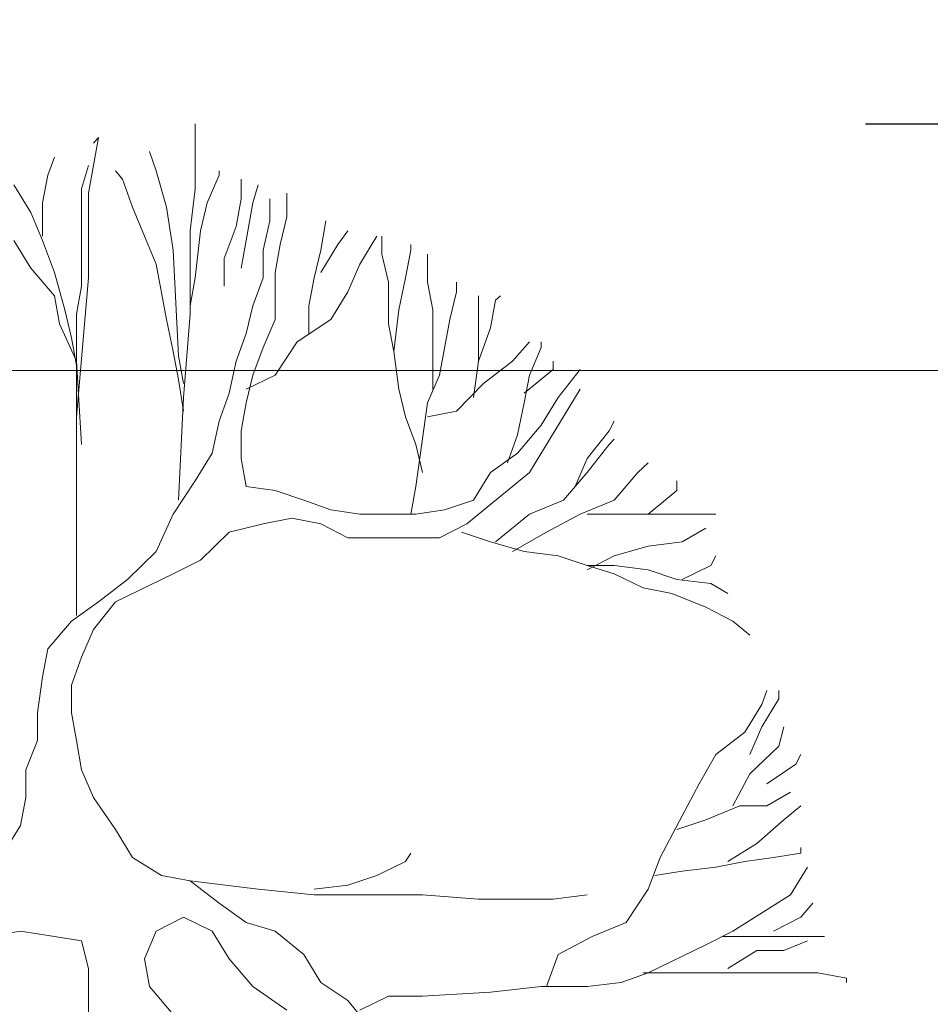
# Model space of a CAD drawing. Units: millimetres. Extents: x 595116 to 630915, y 909473 to 920225.
# Tile 53 of 134: x 629559 to 629589, y 919281 to 919314. Entities that reach past the tile are written whole.
import ezdxf

# ---------------------------------------------------------------- set-up
doc = ezdxf.new("R2010")
doc.units = ezdxf.units.MM
doc.layers.add('Dimension', color=3, linetype='Continuous', lineweight=18)
doc.layers.add('L-PLNT', color=85, linetype='Continuous', lineweight=13)
doc.styles.get("Standard").update_dxf_attribs({"font": 'arial.ttf'})
doc.dimstyles.new('ISO-25', dxfattribs={"dimtxt": 9, "dimasz": 6, "dimexe": 1.25, "dimexo": 0.625, "dimtad": 1, "dimlunit": 4, "dimtxsty": 'Standard', "dimcen": 2.5, "dimadec": 0, "dimazin": 0, "dimtfac": 1, "dimtmove": 0, "dimatfit": 3, "dimfxl": 1, "dimarcsym": 0})

# ---------------------------------------------------------------- blocks, each defined once
blk = doc.blocks.new('A$C143125F4')
for p, q in [((2.883, 4.8338), (2.883, 5.0443)), ((2.5383, 4.8203), (2.5711, 4.9995)), ((2.5711, 4.9995), (2.5547, 4.9816)), ((2.7571, 4.892), (2.7353, 4.9547)), ((2.407, 4.8786), (2.4289, 4.9368)), ((2.5164, 4.8338), (2.5383, 4.9099)), ((2.6477, 4.8651), (2.6259, 4.892)), ((2.79, 4.7755), (2.7571, 4.892)), ((2.9596, 4.8786), (2.9596, 4.892)), ((2.3906, 4.789), (2.407, 4.8786)), ((2.6806, 4.7755), (2.6477, 4.8651)), ((2.9213, 4.789), (2.9596, 4.8786)), ((3.0307, 4.8024), (3.0307, 4.8651)), ((2.3523, 4.7576), (2.2976, 4.8472)), ((2.5164, 4.5202), (2.5164, 4.8338)), ((2.8666, 4.6994), (2.883, 4.8338)), ((3.069, 4.789), (3.0854, 4.8472)), ((2.5383, 4.5471), (2.5383, 4.8203)), ((3.0143, 4.7128), (3.0307, 4.8024)), ((3.1237, 4.7307), (3.1237, 4.8024)), ((3.1784, 4.7442), (3.1784, 4.8203)), ((2.3906, 4.6814), (2.3906, 4.789)), ((2.7189, 4.6814), (2.6806, 4.7755)), ((2.8119, 4.6367), (2.79, 4.7755)), ((2.8994, 4.6994), (2.9213, 4.789)), ((3.0471, 4.668), (3.069, 4.789)), ((2.3906, 4.668), (2.3523, 4.7576)), ((3.1018, 4.6367), (3.1237, 4.7307)), ((3.1565, 4.6546), (3.1784, 4.7442)), ((3.2878, 4.6367), (3.3042, 4.7307)), ((2.8666, 4.4306), (2.8666, 4.6994)), ((2.883, 4.5471), (2.8994, 4.6994)), ((2.976, 4.6098), (3.0143, 4.7128)), ((3.3425, 4.6546), (3.3753, 4.6994)), ((2.3523, 4.5784), (2.2976, 4.668)), ((2.4289, 4.565), (2.3906, 4.668)), ((2.7571, 4.5919), (2.7189, 4.6814)), ((3.0307, 4.5784), (3.0471, 4.668)), ((3.4136, 4.5919), (3.4683, 4.6814)), ((3.4847, 4.6232), (3.4847, 4.6814)), ((2.8283, 4.2962), (2.8119, 4.6367)), ((3.1018, 4.5471), (3.1018, 4.6367)), ((3.1401, 4.565), (3.1565, 4.6546)), ((3.2659, 4.5471), (3.2878, 4.6367)), ((3.2878, 4.565), (3.3425, 4.6546)), ((3.5613, 4.5471), (3.5777, 4.6367)), ((3.5777, 4.6367), (3.5777, 4.6546)), ((2.976, 4.5202), (2.976, 4.6098)), ((3.5066, 4.5336), (3.4847, 4.6232)), ((3.6324, 4.5336), (3.6324, 4.6232)), ((2.4289, 4.4888), (2.3523, 4.5784)), ((2.79, 4.4127), (2.7571, 4.5919)), ((3.3753, 4.5023), (3.4136, 4.5919)), ((2.4617, 4.444), (2.4289, 4.565)), ((2.5, 4.0991), (2.5383, 4.5471)), ((2.8666, 4.4575), (2.883, 4.5471)), ((3.069, 4.4575), (3.1018, 4.5471)), ((3.1401, 4.4127), (3.1401, 4.565)), ((3.2495, 4.4575), (3.2659, 4.5471)), ((3.5394, 4.444), (3.5613, 4.5471)), ((2.5, 4.4306), (2.5164, 4.5202)), ((3.5066, 4.3992), (3.5066, 4.5336)), ((3.6488, 4.444), (3.6324, 4.5336)), ((3.7254, 4.5023), (3.7254, 4.5336)), ((2.4453, 4.3992), (2.4289, 4.4888)), ((3.3206, 4.4127), (3.3753, 4.5023)), ((3.7035, 4.4127), (3.7254, 4.5023)), ((3.7965, 4.2783), (3.7965, 4.4888)), ((3.8512, 4.4754), (3.8677, 4.4888)), ((3.0471, 4.3679), (3.069, 4.4575)), ((3.2495, 4.3679), (3.2495, 4.4575)), ((3.8348, 4.3858), (3.8512, 4.4754)), ((2.4836, 4.3544), (2.4617, 4.444)), ((2.5, 3.4584), (2.5, 4.4306)), ((2.8119, 4.3096), (2.79, 4.4127)), ((2.8447, 4.1618), (2.8666, 4.4306)), ((3.1018, 4.3231), (3.1401, 4.4127)), ((3.2112, 4.341), (3.3206, 4.4127)), ((3.523, 4.3096), (3.5394, 4.444)), ((3.6488, 4.1887), (3.6488, 4.444)), ((3.6707, 4.2335), (3.7035, 4.4127)), ((2.5, 4.2783), (2.4453, 4.3992)), ((3.523, 4.3096), (3.5066, 4.3992)), ((3.7965, 4.2783), (3.8348, 4.3858)), ((2.5, 4.2648), (2.4836, 4.3544)), ((3.0143, 4.2783), (3.0471, 4.3679)), ((3.069, 4.2335), (3.1018, 4.3231)), ((3.1401, 4.2335), (3.2112, 4.341)), ((3.906, 4.2783), (3.9607, 4.341)), ((3.9607, 4.2335), (3.999, 4.3231)), ((3.999, 4.3231), (3.999, 4.341)), ((2.8283, 4.22), (2.8119, 4.3096)), ((2.8447, 4.2066), (2.8283, 4.2962)), ((3.5394, 4.1887), (3.523, 4.3096)), ((2.5164, 4.0095), (2.5, 4.2783)), ((2.9924, 4.1752), (3.0143, 4.2783)), ((3.7801, 4.1618), (3.7965, 4.2783)), ((3.813, 4.2066), (3.906, 4.2783)), ((4.0372, 4.2514), (4.0372, 4.2783)), ((3.0471, 4.1887), (3.1401, 4.2335)), ((3.0471, 4.1439), (3.069, 4.2335)), ((3.6324, 4.1439), (3.6707, 4.2335)), ((3.9442, 4.1752), (4.0372, 4.2514)), ((3.9442, 4.1439), (3.9607, 4.2335)), ((4.1248, 4.2514), (4.0537, 4.1618)), ((2.8447, 4.117), (2.8283, 4.22)), ((3.7254, 4.117), (3.813, 4.2066)), ((2.8283, 3.8303), (2.8447, 4.1618)), ((2.9596, 4.0856), (2.9924, 4.1752)), ((3.5613, 4.0991), (3.5394, 4.1887)), ((3.9607, 3.9199), (4.1248, 4.1887)), ((4.0537, 4.1618), (3.999, 4.0722)), ((3.0307, 4.0543), (3.0471, 4.1439)), ((3.5941, 3.8751), (3.6324, 4.1439)), ((3.9224, 4.0408), (3.9442, 4.1439)), ((2.5, 3.996), (2.5, 4.0991)), ((3.5941, 4.0095), (3.5613, 4.0991)), ((3.6324, 4.0991), (3.7254, 4.117)), ((2.9377, 3.9826), (2.9596, 4.0856)), ((3.999, 4.0722), (3.9224, 3.9826)), ((4.2178, 4.0543), (4.2342, 4.0856)), ((3.0307, 3.9647), (3.0307, 4.0543)), ((3.8895, 3.9512), (3.9224, 4.0408)), ((4.1467, 3.9647), (4.2178, 4.0543)), ((3.616, 3.9199), (3.5941, 4.0095)), ((4.1467, 3.9199), (4.2178, 4.0095)), ((4.2178, 4.0095), (4.2342, 4.0274)), ((2.883, 3.893), (2.9377, 3.9826)), ((3.9224, 3.9826), (3.8348, 3.9199)), ((3.0471, 3.8751), (3.0307, 3.9647)), ((4.1084, 3.8751), (4.1467, 3.9647)), ((4.3108, 3.9199), (4.3436, 3.9512)), ((3.7583, 3.7541), (3.9607, 3.9199)), ((3.8348, 3.9199), (3.7801, 3.8303)), ((4.0701, 3.8303), (4.1467, 3.9199)), ((4.2342, 3.8303), (4.3108, 3.9199)), ((2.8119, 3.7855), (2.883, 3.893)), ((3.1401, 3.8616), (3.0471, 3.8751)), ((3.5777, 3.7855), (3.5941, 3.8751)), ((4.4366, 3.8616), (4.4366, 3.893)), ((3.2331, 3.8303), (3.1401, 3.8616)), ((4.3436, 3.7855), (4.4366, 3.8616)), ((3.3206, 3.7989), (3.2331, 3.8303)), ((3.7801, 3.8303), (3.6871, 3.7989)), ((3.9607, 3.7855), (4.0701, 3.8303)), ((4.1248, 3.7855), (4.2342, 3.8303)), ((2.7571, 3.6645), (2.8119, 3.7855)), ((3.4136, 3.7855), (3.3206, 3.7989)), ((3.5941, 3.7855), (3.4136, 3.7855)), ((3.6871, 3.7989), (3.5941, 3.7855)), ((3.8512, 3.6959), (3.9607, 3.7855)), ((4.0154, 3.7272), (4.1248, 3.7855)), ((4.1467, 3.7855), (4.5624, 3.7855)), ((2.9924, 3.7272), (3.1018, 3.7541)), ((3.1018, 3.7541), (3.1948, 3.772)), ((3.1948, 3.772), (3.2878, 3.7541)), ((3.2878, 3.7541), (3.3753, 3.7093)), ((3.6707, 3.7093), (3.7583, 3.7541)), ((2.8994, 3.6376), (2.9924, 3.7272)), ((3.7418, 3.7272), (3.8348, 3.6959)), ((3.906, 3.6645), (4.0154, 3.7272)), ((4.453, 3.6959), (4.5296, 3.7407)), ((3.3753, 3.7093), (3.6707, 3.7093)), ((3.8348, 3.6959), (3.9442, 3.6645)), ((4.2342, 3.6511), (4.3436, 3.6824)), ((4.3436, 3.6824), (4.453, 3.6959)), ((2.6641, 3.5749), (2.7571, 3.6645)), ((3.9442, 3.6645), (4.0537, 3.6511)), ((4.0537, 3.6511), (4.1467, 3.6197)), ((4.1467, 3.6063), (4.2342, 3.6511)), ((4.546, 3.6197), (4.5624, 3.6511)), ((2.8119, 3.5928), (2.8994, 3.6376)), ((4.1467, 3.6197), (4.2342, 3.5928)), ((4.1467, 3.6197), (4.2342, 3.6197)), ((4.2342, 3.6197), (4.3436, 3.6063)), ((4.453, 3.5749), (4.546, 3.6197)), ((2.6259, 3.5032), (2.8119, 3.5928)), ((4.2342, 3.5928), (4.3272, 3.548)), ((4.3436, 3.6063), (4.4366, 3.5749)), ((2.5711, 3.5032), (2.6641, 3.5749)), ((4.4366, 3.5749), (4.546, 3.5615)), ((4.546, 3.5615), (4.6007, 3.5301)), ((4.3272, 3.548), (4.4202, 3.5301)), ((4.4202, 3.5301), (4.5296, 3.4853)), ((2.4836, 3.4405), (2.5711, 3.5032)), ((2.5547, 3.4136), (2.6259, 3.5032)), ((4.5296, 3.4853), (4.6171, 3.4405)), ((2.407, 3.3509), (2.4836, 3.4405)), ((4.6171, 3.4405), (4.6718, 3.3957)), ((2.5164, 3.3241), (2.5547, 3.4136)), ((2.3906, 3.2613), (2.407, 3.3509)), ((2.4836, 3.2345), (2.5164, 3.3241)), ((2.3742, 3.1449), (2.3906, 3.2613)), ((2.4836, 3.1449), (2.4836, 3.2345)), ((4.7101, 3.1717), (4.7265, 3.2165)), ((4.7648, 3.1897), (4.7648, 3.2165)), ((4.7101, 3.1001), (4.7648, 3.1897)), ((2.3742, 3.0553), (2.3742, 3.1449)), ((2.5, 3.0553), (2.4836, 3.1449)), ((4.6554, 3.0821), (4.7101, 3.1717)), ((4.5624, 3.0105), (4.6554, 3.0821)), ((4.6718, 3.0105), (4.7101, 3.1001)), ((4.7648, 3.0373), (4.7812, 3.1001)), ((2.3359, 2.9612), (2.3742, 3.0553)), ((2.5164, 2.9612), (2.5, 3.0553)), ((4.6718, 2.9477), (4.7648, 3.0373)), ((4.5077, 2.9164), (4.5624, 3.0105)), ((4.8195, 2.9791), (4.8359, 3.0105)), ((2.3359, 2.8716), (2.3359, 2.9612)), ((2.5547, 2.8716), (2.5164, 2.9612)), ((4.7265, 2.9164), (4.8195, 2.9791)), ((4.6171, 2.8447), (4.6718, 2.9477)), ((4.453, 2.8133), (4.5077, 2.9164)), ((4.7265, 2.8447), (4.8031, 2.8895)), ((2.3195, 2.782), (2.3359, 2.8716)), ((2.6259, 2.7686), (2.5547, 2.8716)), ((4.5296, 2.7999), (4.639, 2.8447)), ((4.639, 2.8447), (4.7265, 2.8447)), ((4.7812, 2.7999), (4.8359, 2.8447)), ((4.3819, 2.679), (4.453, 2.8133)), ((4.4366, 2.7686), (4.5296, 2.7999)), ((4.6937, 2.7238), (4.7812, 2.7999)), ((2.2648, 2.6924), (2.3195, 2.782)), ((2.6806, 2.679), (2.6259, 2.7686)), ((4.6007, 2.6655), (4.6937, 2.7238)), ((4.8359, 2.6924), (4.8359, 2.7103)), ((2.7736, 2.6207), (2.6806, 2.679)), ((3.5613, 2.6655), (3.5777, 2.6924)), ((4.3436, 2.5759), (4.3819, 2.679)), ((4.6554, 2.6655), (4.7484, 2.679)), ((4.7484, 2.679), (4.8359, 2.6924)), ((3.4683, 2.6207), (3.5613, 2.6655)), ((4.453, 2.6342), (4.5624, 2.6476)), ((4.5624, 2.6476), (4.6554, 2.6655)), ((4.8031, 2.558), (4.8578, 2.6476)), ((2.8666, 2.6028), (2.7736, 2.6207)), ((3.3753, 2.5894), (3.4683, 2.6207)), ((4.3655, 2.6207), (4.453, 2.6342)), ((2.8666, 2.6028), (3.0854, 2.5759)), ((2.9596, 2.5311), (2.8666, 2.6028)), ((3.0854, 2.5759), (3.2659, 2.558)), ((3.2659, 2.5759), (3.3753, 2.5894)), ((4.2725, 2.4684), (4.3436, 2.5759)), ((3.2659, 2.558), (3.616, 2.558)), ((3.616, 2.558), (3.7965, 2.5446)), ((3.7965, 2.5446), (4.0372, 2.5446)), ((4.0372, 2.5446), (4.1467, 2.558)), ((4.6171, 2.4415), (4.8031, 2.558)), ((3.0471, 2.4684), (2.9596, 2.5311)), ((4.8359, 2.4863), (4.8742, 2.5311)), ((2.8447, 2.4863), (2.7571, 2.4415)), ((2.9377, 2.4415), (2.8447, 2.4863)), ((4.7484, 2.4415), (4.8359, 2.4863)), ((3.1401, 2.4415), (3.0471, 2.4684)), ((4.1631, 2.4236), (4.2725, 2.4684)), ((2.3195, 2.4415), (2.2101, 2.4236)), ((2.4289, 2.4236), (2.3195, 2.4415)), ((2.5164, 2.4102), (2.4289, 2.4236)), ((2.7571, 2.4415), (2.7189, 2.3519)), ((2.9924, 2.3519), (2.9377, 2.4415)), ((3.2331, 2.3654), (3.1401, 2.4415)), ((4.0537, 2.3654), (4.1631, 2.4236)), ((4.5296, 2.3967), (4.6171, 2.4415)), ((4.5843, 2.4236), (4.9125, 2.4236)), ((2.5383, 2.3206), (2.5164, 2.4102)), ((4.3436, 2.3071), (4.5296, 2.3967)), ((4.7812, 2.3788), (4.8578, 2.4102)), ((2.7189, 2.3519), (2.7353, 2.2623)), ((3.069, 2.2623), (2.9924, 2.3519)), ((3.2878, 2.2758), (3.2331, 2.3654)), ((4.0154, 2.2623), (4.0537, 2.3654)), ((4.6007, 2.3206), (4.6937, 2.3788)), ((4.6937, 2.3788), (4.7812, 2.3788)), ((2.5383, 1.8726), (2.5383, 2.3206)), ((4.2561, 2.2758), (4.3436, 2.3071)), ((4.3272, 2.3071), (4.8906, 2.3071)), ((4.8906, 2.3071), (4.9836, 2.2892)), ((4.9836, 2.2892), (4.9836, 2.2758)), ((2.7353, 2.2623), (2.8119, 2.1727)), ((3.1784, 2.1862), (3.069, 2.2623)), ((3.3753, 2.2175), (3.2878, 2.2758)), ((3.8348, 2.2444), (3.999, 2.2623)), ((3.999, 2.2623), (4.1467, 2.2623)), ((4.1467, 2.2623), (4.2561, 2.2758)), ((3.4136, 2.1862), (3.5066, 2.231)), ((3.5066, 2.231), (3.616, 2.231)), ((3.616, 2.231), (3.8348, 2.2444)), ((3.4519, 2.1235), (3.3753, 2.2175))]:
    blk.add_line(p, q)
blk = doc.blocks.new('*D210')
at = {"layer": 'Defpoints', "color": 0, "transparency": 16777216}
for p in [(629586.227, 919310.123), (629593.946, 919310.123), (629586.227, 919258.662)]:
    blk.add_point(p, dxfattribs=at)
at = {"layer": 'Dimension', "color": 0, "lineweight": -2, "transparency": 16777216}
for p, q in [((629593.946, 919310.123), (629593.946, 919449.69)), ((629586.852, 919310.123), (629595.196, 919310.123)), ((629593.946, 919264.662), (629593.946, 919304.123)), ((629586.852, 919258.662), (629595.196, 919258.662))]:
    blk.add_line(p, q, dxfattribs=at)
at = {"layer": 'Dimension', "color": 0, "transparency": 16777216}
for points in [[(629592.946, 919304.123), (629594.946, 919304.123), (629593.946, 919310.123)], [(629592.946, 919264.662), (629594.946, 919264.662), (629593.946, 919258.662)]]:
    blk.add_solid(points, dxfattribs=at)
at = {"layer": 'Dimension', "color": 0, "transparency": 16777216, "insert": (629588.662, 919382.907), "char_height": 9, "attachment_point": 5, "rotation": 90}
blk.add_mtext('CANOPY 4\'-3 1/2" TYP.', dxfattribs=at)
blk = doc.blocks.new('*D216')
at = {"layer": 'Defpoints', "color": 0, "transparency": 16777216}
for p in [(629743.541, 919411.928), (629505.041, 919411.828), (629743.541, 918832.378)]:
    blk.add_point(p, dxfattribs=at)
at = {"layer": 'Dimension', "color": 0, "lineweight": -2, "transparency": 16777216}
for p, q in [((629743.541, 919411.303), (629743.541, 918831.128)), ((629505.041, 919411.203), (629505.041, 918831.128)), ((629511.041, 918832.378), (629737.541, 918832.378))]:
    blk.add_line(p, q, dxfattribs=at)
at = {"layer": 'Dimension', "color": 0, "transparency": 16777216}
for points in [[(629511.041, 918833.378), (629511.041, 918831.378), (629505.041, 918832.378)], [(629737.541, 918833.378), (629737.541, 918831.378), (629743.541, 918832.378)]]:
    blk.add_solid(points, dxfattribs=at)
at = {"layer": 'Dimension', "color": 0, "transparency": 16777216, "insert": (629624.291, 918837.656), "char_height": 9, "attachment_point": 5}
blk.add_mtext('19\'-10 1/2"', dxfattribs=at)
blk = doc.blocks.new('*D220')
at = {"layer": 'Defpoints', "color": 0, "transparency": 16777216}
for p in [(629824.951, 920160.756), (629511.274, 919302.009), (629824.951, 919302.009)]:
    blk.add_point(p, dxfattribs=at)
at = {"layer": 'Dimension', "color": 0, "lineweight": -2, "transparency": 16777216}
for p, q in [((629511.274, 919302.634), (629511.274, 920162.006)), ((629824.951, 919302.634), (629824.951, 920162.006)), ((629517.274, 920160.756), (629818.951, 920160.756))]:
    blk.add_line(p, q, dxfattribs=at)
at = {"layer": 'Dimension', "color": 0, "transparency": 16777216}
for points in [[(629517.274, 920161.756), (629517.274, 920159.756), (629511.274, 920160.756)], [(629818.951, 920161.756), (629818.951, 920159.756), (629824.951, 920160.756)]]:
    blk.add_solid(points, dxfattribs=at)
at = {"layer": 'Dimension', "color": 0, "transparency": 16777216, "insert": (629668.113, 920166.035), "char_height": 9, "attachment_point": 5}
blk.add_mtext('26\'-1 1/2"', dxfattribs=at)

msp = doc.modelspace()

# ---------------------------------------------------------------- linework, layer by layer
at = {"layer": 'L-PLNT'}
msp.add_line((629824.951, 919302.009), (629511.274, 919302.009), dxfattribs=at)

# ---------------------------------------------------------------- block references
at = {"layer": 'L-PLNT', "xscale": 10.20167662382051, "yscale": 10.20167662382051, "zscale": 10.20167662382051}
msp.add_blockref('A$C143125F4', (629535.386, 919258.662), dxfattribs=at)

# ---------------------------------------------------------------- dimensions: what is measured, and where the dimension line sits
at = {"layer": 'Dimension'}
for base, p1, p2, picture, middle in [((629824.951, 920160.756), (629511.274, 919302.009), (629824.951, 919302.009), '*D220', (629668.113, 920166.035)), ((629743.541, 918832.378), (629505.041, 919411.828), (629743.541, 919411.928), '*D216', (629624.291, 918837.656))]:
    dim = msp.add_linear_dim(base=base, p1=p1, p2=p2, dimstyle='ISO-25', override={"dimdec": 1, "dimlfac": 1, "dimrnd": 0, "dimzin": 1, "dimdsep": 46, "dimlunit": 4, "dimfrac": 2}, dxfattribs=at)
    dim.commit()
    dim.dimension.update_dxf_attribs({"geometry": picture, "text_midpoint": middle})
dim = msp.add_linear_dim(base=(629593.946, 919310.123), p1=(629586.227, 919258.662), p2=(629586.227, 919310.123), angle=90, text='CANOPY <> TYP.', dimstyle='ISO-25', override={"dimdec": 1, "dimlfac": 1, "dimrnd": 0, "dimzin": 1, "dimdsep": 46, "dimlunit": 4, "dimfrac": 2}, dxfattribs=at)
dim.commit()
dim.dimension.update_dxf_attribs({"geometry": '*D210', "text_midpoint": (629588.662, 919382.907)})

doc.saveas('drawing.dxf')
